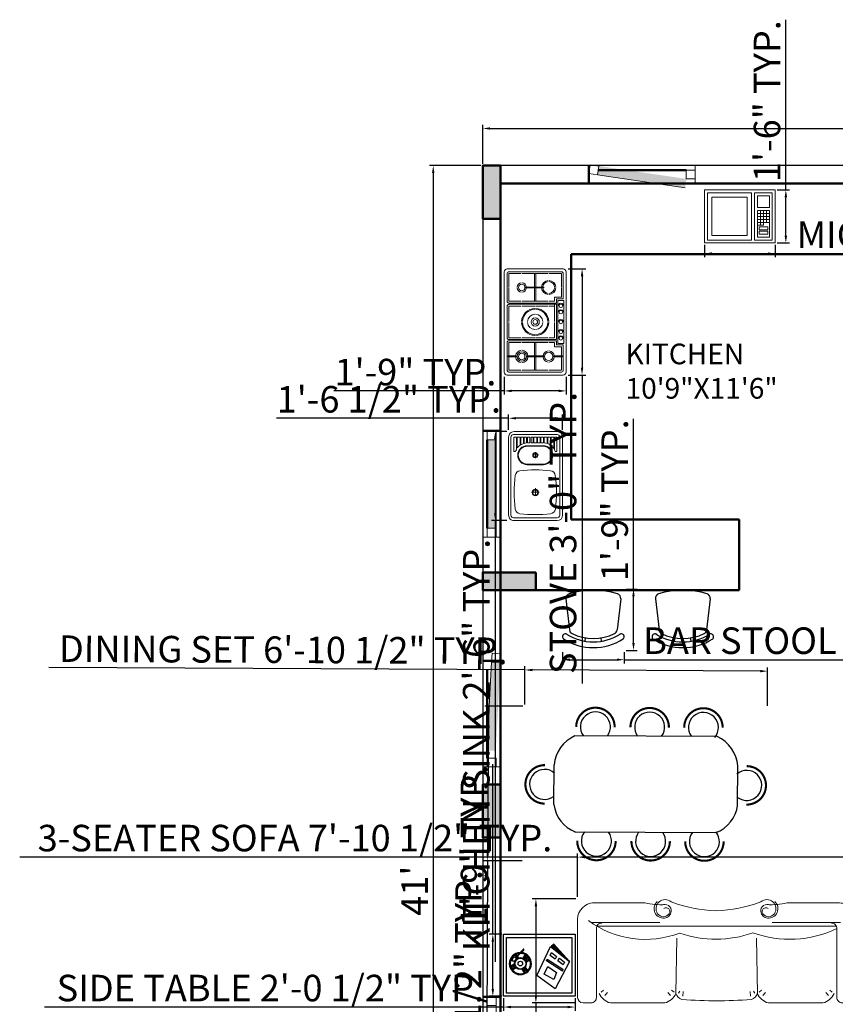
# Model space of a CAD drawing. Units: inches. Extents: x 3064 to 19385, y 846 to 15425.
# Tile 3 of 108: x 3064 to 3340, y 1112 to 1446. Entities that reach past the tile are written whole.
import ezdxf

# ---------------------------------------------------------------- set-up
doc = ezdxf.new("R2010")
doc.units = ezdxf.units.IN
for name, color, linetype, lineweight in [('A-ANNO-DIMS', 2, 'Continuous', 18), ('A-AREA-IDEN', 3, 'Continuous', 18), ('A-COLS', 1, 'Continuous', 35), ('A-EQPM', 8, 'Continuous', 18), ('A-FLOR-FIXT', 9, 'Continuous', 18), ('A-FURN', 8, 'Continuous', 18), ('A-GLAZ', 4, 'Continuous', 18), ('A-WALL', 7, 'Continuous', 50), ('C-PROP', 6, 'Continuous', 25)]:
    doc.layers.add(name, color=color, linetype=linetype, lineweight=lineweight)
for name, color, linetype in [('BLO', 135, 'Continuous'), ('FUR', 42, 'Continuous'), ('NOITHAT', 21, 'Continuous'), ('Win', 152, 'Continuous')]:
    doc.layers.add(name, color=color, linetype=linetype)
doc.styles.get("Standard").update_dxf_attribs({"font": 'arial.ttf'})
doc.dimstyles.new('ISO-25', dxfattribs={"dimtxt": 9, "dimasz": 2.5, "dimexe": 1.25, "dimexo": 0.625, "dimtad": 1, "dimdec": 1, "dimlunit": 3, "dimtxsty": 'Standard', "dimcen": 2.5, "dimadec": 0, "dimazin": 0, "dimtfac": 1, "dimtdec": 1, "dimtmove": 0, "dimatfit": 3, "dimfxl": 1, "dimarcsym": 0})

# ---------------------------------------------------------------- blocks, each defined once
blk = doc.blocks.new('din')
at = {"layer": 'FUR', "ltscale": 0.25}
for p, q in [((70.23, 15.24), (9.28, 15.24)), ((0, 3.44), (0, -13.56)), ((79.14, 3.44), (79.14, -13.56)), ((8.91, -26.16), (70.23, -26.16))]:
    blk.add_line(p, q, dxfattribs=at)
at = {"layer": 'FUR', "ltscale": 0.25, "const_width": 0.9}
for points in [[(22.5, 19.02, 1.012537), (5.94, 19.02, 1.012537)], [(45.67, 19.02, 1.012537), (29.11, 19.02, 1.012537)], [(69.02, 19.02, 1.012537), (52.46, 19.02, 1.012537)], [(-3.79, 3.1, 1.012537), (-3.79, -13.47, 1.012537)], [(83.08, 3.1, -1.012537), (83.08, -13.47, -1.012537)], [(23.18, -29.95, -1.012537), (6.61, -29.95, -1.012537)], [(46.34, -29.95, -1.012537), (29.78, -29.95, -1.012537)], [(69.7, -29.95, -1.012537), (53.14, -29.95, -1.012537)]]:
    blk.add_lwpolyline(points, format="xyb", dxfattribs=at)
at = {"layer": 'FUR', "ltscale": 0.25}
for centre, radius, start, end in [((14.22, 19.13), 6.48, 323.1301, 221.2163), ((37.39, 19.13), 6.48, 323.1301, 216.8699), ((60.74, 19.13), 6.48, 323.1301, 216.8699), ((14.55, 1.54), 14.67, 111.0491, 172.5731), ((64.59, 1.54), 14.67, 7.4269, 68.9509), ((-3.89, -5.18), 6.48, 53.1301, 311.2163), ((83.18, -5.18), 6.48, 228.7837, 126.8699), ((15.28, -12.21), 15.34, 185.0602, 245.4675), ((63.86, -12.21), 15.34, 294.5325, 354.9398), ((14.89, -30.05), 6.48, 138.7837, 36.8699), ((38.06, -30.05), 6.48, 143.1301, 36.8699), ((61.42, -30.05), 6.48, 143.1301, 36.8699)]:
    blk.add_arc(centre, radius, start, end, dxfattribs=at)
blk = doc.blocks.new('A$C558E769F')
at = {"layer": 'NOITHAT'}
for p, q in [((29.4, 426.4), (61.1, 154.1)), ((508.9, 426.4), (477.2, 154.1)), ((197.1, 55.9), (201.8, 84.2)), ((341.2, 55.9), (336.5, 84.2))]:
    blk.add_line(p, q, dxfattribs=at)
for centre, radius, start, end in [((69.1, 431), 40, 107.02981, 186.63805), ((269.2, -222), 723, 72.97019, 107.02981), ((469.2, 431), 40, 353.36195, 72.97019), ((25.3, 93.7), 25.7, 44.80366, 252.32262), ((269.2, 492.6), 442.6, 237.77056, 302.22944), ((100.8, 158.7), 40, 186.63805, 243.24485), ((269.2, 492.6), 413.9, 243.24485, 296.75515), ((437.5, 158.7), 40, 296.75515, 353.36195), ((513, 93.7), 25.7, 287.67738, 135.19634), ((269.2, 492.6), 492.6, 237.85101, 302.14899)]:
    blk.add_arc(centre, radius, start, end, dxfattribs=at)
blk = doc.blocks.new('sofa-32')
at = {"color": 0, "linetype": 'ByBlock'}
for p, q in [((-0.026, 0.9238), (-0.1, 0.9238)), ((0.657, 0.9252), (0.1531, 0.9252)), ((1.6158, 0.9252), (2.1197, 0.9252)), ((2.3728, 0.9238), (2.2988, 0.9238)), ((-0.15, 0.15), (-0.15, 0.8738)), ((0.024, 0.2361), (0.024, 0.8738)), ((0.05, 0.8375), (0.05, 0.8379)), ((0.0903, 0.8062), (0.0682, 0.8242)), ((0.1006, 0.8574), (0.1265, 0.8286)), ((0.7096, 0.8574), (0.6837, 0.8286)), ((0.7199, 0.8062), (0.742, 0.8242)), ((0.7682, 0.3257), (0.7597, 0.8384)), ((0.7601, 0.8375), (0.7601, 0.8379)), ((0.7823, 0.8346), (0.7966, 0.8162)), ((0.8227, 0.8633), (0.8259, 0.8195)), ((1.4501, 0.8633), (1.447, 0.8195)), ((1.4906, 0.8346), (1.4762, 0.8162)), ((1.5046, 0.3257), (1.5131, 0.8384)), ((1.5127, 0.8375), (1.5127, 0.8379)), ((1.5529, 0.8062), (1.5308, 0.8242)), ((1.5632, 0.8574), (1.5891, 0.8286)), ((2.1722, 0.8574), (2.1463, 0.8286)), ((2.1825, 0.8062), (2.2046, 0.8242)), ((2.2228, 0.8375), (2.2228, 0.8379)), ((2.2228, 0.8375), (2.2228, 0.8379)), ((2.2488, 0.2361), (2.2488, 0.8738)), ((2.4228, 0.15), (2.4228, 0.8738)), ((0.0289, 0.2145), (2.2439, 0.2145)), ((-0.01, 0.1801), (0.6238, 0.1801)), ((2.2948, 0.1801), (1.661, 0.1801)), ((0, 0), (0.4856, 0)), ((2.2848, 0), (1.7991, 0))]:
    blk.add_line(p, q, dxfattribs=at)
at = {"color": 0, "linetype": 'ByBlock', "extrusion": (0, 0, -1)}
for centre, major_axis, start_param, end_param in [((-0.1, 0.8738), (0.0354, 0.0354), 3.926992, 5.497787), ((-0.026, 0.8738), (-0.0354, 0.0354), 0.785398, 2.356196), ((0.1997, 0.7661), (0.1173, 0.1173), 4.372209, 5.213218), ((0.6105, 0.7661), (0.1173, 0.1173), -0.500829, 0.34018), ((1.6624, 0.7661), (0.1173, 0.1173), 4.372209, 5.213218), ((2.0731, 0.7661), (-0.1173, 0.1173), 1.069968, 1.910976), ((2.2988, 0.8738), (-0.0354, 0.0354), 5.497786, 7.068583), ((2.3728, 0.8738), (0.0354, 0.0354), -0.785398, 0.785398), ((0.8378, 0.8143), (-0.0573, 0.0573), 5.78837, 6.779907), ((1.1202, -2.7856), (2.6094, 2.6094), -0.86827, -0.778364), ((1.1526, -2.7856), (2.6094, 2.6094), -0.792432, -0.702526), ((1.435, 0.8143), (-0.0573, 0.0573), 1.074075, 2.065611), ((0.4599, -0.6685), (0.71, 0.71), 5.048761, 5.844539), ((1.7954, -0.5466), (-0.6249, 0.6249), 0.417642, 1.423136), ((1.1424, -0.6685), (-0.71, 0.71), 0.438646, 1.125824), ((0.074, 0.2361), (0.0354, 0.0354), 2.356194, 3.926992), ((2.1988, 0.2361), (0.0354, 0.0354), 0.785397, 2.356194), ((0, 0.15), (0.1061, 0.1061), 2.356194, 3.926992), ((0.6576, 0.0525), (-0.0624, 0.0624), 4.675944, 7.152385), ((0.6708, 0.0524), (-0.059, 0.059), 3.186406, 6.094039), ((0.6552, 0.0629), (0.0458, 0.0458), 4.523242, 6.472337), ((0.6801, 0.0798), (-0.0245, 0.0245), 1.759948, 4.523241), ((0.6592, 0.0712), (-0.0491, 0.0491), 0.8692, 2.230507), ((1.6256, 0.0712), (-0.0491, 0.0491), 5.623477, 6.984784), ((1.614, 0.0524), (0.059, 0.059), 0.189149, 3.096782), ((1.6047, 0.0798), (0.0245, 0.0245), 1.759947, 4.52324), ((1.6295, 0.0629), (0.0458, 0.0458), 4.52324, 6.472335), ((1.6271, 0.0525), (-0.0624, 0.0624), 0.701599, 3.17804), ((2.2728, 0.15), (0.1061, 0.1061), 0.785398, 2.356194), ((0.6324, -0.6613), (-0.479, 0.479), 0.566947, 0.842011), ((0.6701, 0.0726), (0.0414, 0.0414), 0.659711, 2.852687), ((1.2153, -1.3904), (1.0359, 1.0359), 5.158011, 5.447964), ((1.0694, -1.3904), (1.0359, 1.0359), 5.547613, 5.837566), ((1.6147, 0.0726), (-0.0414, 0.0414), 3.430501, 5.623477), ((1.6523, -0.6613), (0.479, 0.479), 5.441177, 5.716241)]:
    blk.add_ellipse(centre, major_axis=major_axis, ratio=1, start_param=start_param, end_param=end_param, dxfattribs=at)
blk = doc.blocks.new('sink 1')
for points in [[(5.86, 24.22), (-5.86, 24.22)], [(-7.34, 1.48), (-7.34, 22.73)], [(-6.56, 1.48), (-6.56, 22.73)], [(6.01, 23.43), (-5.86, 23.43)], [(6.72, 1.48), (6.72, 22.73)], [(7.34, 1.48), (7.34, 22.73)], [(1.09, 16.48), (-0.94, 16.48)], [(0, 15.39), (0, 17.42)], [(-2.09, 8.99), (2.28, 8.99)], [(-2.09, 8.84), (2.28, 8.84)], [(-5.78, 5.39), (-5.78, 5.39)], [(-5.31, 5.39), (-5.31, 5.39)], [(0.78, 6.33), (-0.78, 6.33)], [(0, 5.55), (0, 7.26)], [(5.94, 5.39), (5.94, 5.39)], [(-5.16, 4.92), (-5.16, 4.92)], [(-5, 1.48), (-5, 4.69)], [(-5, 1.48), (-4.22, 1.48), (-4.22, 3.83)], [(-4.84, 4.45), (-4.84, 4.45)], [(-4.22, 3.83), (-4.22, 3.83)], [(-4.06, 1.48), (-4.06, 3.69)], [(-4.06, 1.48), (-3.28, 1.48), (-3.28, 3.27)], [(-3.91, 3.52), (-3.91, 3.52)], [(-3.28, 3.2), (-3.28, 3.2)], [(-3.12, 3.2), (-3.12, 3.2)], [(-2.34, 3.05), (-2.34, 3.05)], [(-2.19, 3.05), (-2.19, 3.05)], [(-2.09, 3.99), (2.28, 3.99)], [(-2.09, 3.84), (2.28, 3.84)], [(-1.41, 3.05), (-1.41, 3.05)], [(-1.25, 3.05), (-1.25, 3.05)], [(-0.47, 1.48), (-1.25, 1.48), (-1.25, 3.05), (-0.47, 3.05)], [(-0.62, 3.05), (-0.62, 3.05)], [(-0.47, 1.48), (-0.47, 3.05)], [(-0.31, 3.05), (-0.31, 3.05)], [(0.47, 1.48), (-0.31, 1.48), (-0.31, 3.05), (0.47, 3.05)], [(0.31, 3.05), (0.31, 3.05)], [(0.47, 1.48), (0.47, 3.05)], [(0.62, 3.05), (0.62, 3.05)], [(1.25, 3.05), (1.25, 3.05)], [(1.56, 3.05), (1.56, 3.05)], [(2.19, 3.05), (2.19, 3.05)], [(2.5, 3.05), (2.5, 3.05)], [(3.12, 3.2), (3.12, 3.2)], [(3.28, 1.48), (4.06, 1.48), (4.06, 3.57)], [(3.28, 1.48), (3.28, 3.2)], [(3.44, 3.2), (3.44, 3.2)], [(4.06, 3.52), (4.06, 3.52)], [(4.22, 1.48), (4.22, 3.67)], [(4.37, 3.83), (4.37, 3.83)], [(5, 4.45), (5, 4.45)], [(5.16, 4.92), (5.16, 4.92)], [(6.01, 0.78), (-5.86, 0.78)], [(5.86, 0), (-5.86, 0)], [(-5.78, 1.48), (-5.78, 1.48)], [(-5.16, 1.48), (-5.16, 1.48)], [(-4.84, 1.48), (-4.84, 1.48)], [(-4.22, 1.48), (-4.22, 1.48)], [(-3.91, 1.48), (-3.91, 1.48)], [(-3.28, 1.48), (-3.28, 1.48)], [(-3.12, 1.48), (-3.12, 1.48)], [(-2.34, 1.48), (-2.34, 1.48)], [(-2.19, 1.48), (-2.19, 1.48)], [(-1.41, 1.48), (-1.41, 1.48)], [(-1.25, 1.48), (-1.25, 1.48)], [(-0.62, 1.48), (-0.62, 1.48)], [(-0.31, 1.48), (-0.31, 1.48)], [(0.31, 1.48), (0.31, 1.48)], [(0.62, 1.48), (0.62, 1.48)], [(1.25, 1.48), (1.25, 1.48)], [(1.56, 1.48), (1.56, 1.48)], [(2.19, 1.48), (2.19, 1.48)], [(2.5, 1.48), (2.5, 1.48)], [(3.12, 1.48), (3.12, 1.48)], [(3.44, 1.48), (3.44, 1.48)], [(4.06, 1.48), (4.06, 1.48)], [(4.37, 1.48), (4.37, 1.48)], [(5, 1.48), (5, 1.48)], [(5.16, 1.48), (5.16, 1.48)], [(5.94, 1.48), (5.94, 1.48)]]:
    blk.add_lwpolyline(points)
for points in [[(-5.16, 4.92), (-5.16, 1.48), (-5.78, 1.48), (-5.78, 5.39), (-5.31, 5.39, -0.068511), (-5.16, 4.92)], [(5.16, 4.92, 0.248301), (5.47, 5.39), (5.94, 5.39), (5.94, 1.48), (5.16, 1.48), (5.16, 4.92)], [(4.06, 3.57, -0.061679), (3.32, 3.22)], [(4.22, 1.48), (5, 1.48), (5, 4.45, -0.083542), (4.22, 3.67, -0.083542)]]:
    blk.add_lwpolyline(points, format="xyb")
for points in [[(-3.12, 3.22), (-3.12, 1.48), (-2.34, 1.48), (-2.34, 3.05, -0.06228)], [(2.5, 3.05), (2.5, 1.48), (3.12, 1.48), (3.12, 3.2, -0.050256)]]:
    blk.add_lwpolyline(points, format="xyb", close=True)
for points in [[(-2.19, 3.05), (-1.41, 3.05), (-1.41, 1.48), (-2.19, 1.48)], [(0.62, 3.05), (1.25, 3.05), (1.25, 1.48), (0.62, 1.48)], [(2.19, 1.48), (2.19, 3.05), (1.56, 3.05), (1.56, 1.48)]]:
    blk.add_lwpolyline(points, close=True)
for centre, radius in [((0.09, 16.57), 0.859), ((0.09, 16.57), 0.703), ((0.09, 6.41), 0.703), ((0.09, 6.41), 0.547)]:
    blk.add_circle(centre, radius)
for centre, radius, start, end in [((-5.86, 22.73), 1.48, 90, 180), ((5.86, 22.73), 1.48, 360, 90), ((-5.86, 22.73), 0.703, 90, 180), ((-3.87, 20.82), 1.53, 97.3256, 171.1849), ((0.09, -12.65), 35.23, 83.2159, 96.7841), ((4.06, 20.82), 1.53, 8.8151, 82.6744), ((6.01, 22.73), 0.703, 0, 90), ((30.19, 16.56), 35.85, 172.7947, 187.4213), ((-30, 16.56), 35.85, 352.5787, 7.2053), ((-3.89, 12.12), 1.48, 187.4212, 263.2159), ((4.08, 12.12), 1.48, 276.7841, 352.5788), ((-2.1, 6.41), 2.58, 90, 270), ((-2.1, 6.41), 2.42, 90, 270), ((0.09, 45.63), 35.23, 263.2159, 276.7841), ((2.28, 6.41), 2.58, 270, 90), ((2.28, 6.41), 2.42, 270, 90), ((-2.15, 6.48), 3.36, 212.1095, 232.0862), ((-2.1, 6.41), 3.36, 234.156, 249.3275), ((2.14, 6.36), 3.36, 289.8633, 290.5971), ((-5.86, 1.48), 1.48, 180, 270), ((-5.86, 1.48), 0.703, 180, 270), ((5.86, 1.48), 1.48, 270, 0), ((6.01, 1.48), 0.703, 270, 360)]:
    blk.add_arc(centre, radius, start, end)
blk = doc.blocks.new('STOVE')
for p, q in [((11.85, 19.7), (11.55, 19.7)), ((11.55, 16.92), (11.55, 19.7)), ((11.85, 16.92), (11.55, 16.92)), ((11.85, 16.92), (11.85, 19.7)), ((-11.85, 13.73), (-11.85, 7.62)), ((-11.85, 13.73), (-11.55, 13.73)), ((-11.55, 13.73), (-11.55, 7.62)), ((-11.85, 10.75), (-16.4, 10.75)), ((-11.85, 10.25), (-16.4, 10.25)), ((-7, 10.75), (-11.55, 10.75)), ((-7, 10.25), (-11.55, 10.25)), ((7, 10.75), (11.55, 10.75)), ((7, 10.25), (11.55, 10.25)), ((11.85, 13.23), (11.55, 13.23)), ((11.55, 13.23), (11.55, 7.57)), ((11.85, 13.23), (11.85, 7.57)), ((11.85, 10.75), (16.4, 10.75)), ((11.85, 10.25), (16.4, 10.25)), ((-11.85, 7.62), (-11.55, 7.62)), ((11.85, 7.57), (11.55, 7.57)), ((-7, 3.9), (-8.4, 3.9)), ((-5.4, 3.9), (-6, 3.9)), ((-5.4, 3.9), (-0.15, 3.9)), ((0.15, 3.9), (5.4, 3.9)), ((7, 3.9), (8.4, 3.9)), ((8.4, 3.9), (8.4, 1.6)), ((11.85, 4.28), (11.55, 4.28)), ((11.55, 4.28), (11.55, 1.3)), ((11.85, 4.28), (11.85, 1.3)), ((-7.8, 3.3), (-7.8, 1)), ((-6.4, 3.3), (-7.8, 3.3)), ((7.3, 2.8), (-7.3, 2.8)), ((-7.3, 2.8), (-7.3, 0.8)), ((7.3, 0.8), (-7.3, 0.8)), ((6.4, 3.3), (7.8, 3.3)), ((7.3, 2.8), (7.3, 0.8)), ((7.8, 3.3), (7.8, 1)), ((11.85, 1.3), (11.55, 1.3))]:
    blk.add_line(p, q)
for points in [[(-17, 21), (17, 21, -0.414214), (18, 20), (18, 1, -0.414214), (17, 0), (-17, 0, -0.414214), (-18, 1), (-18, 20, -0.414214)], [(6, 3.3), (-6, 3.3), (-6, 19.4, -0.414214), (-5.4, 20), (5.4, 20, -0.414214), (6, 19.4)]]:
    blk.add_lwpolyline(points, format="xyb", close=True)
for points in [[(-7.8, 1), (-16.4, 1, -0.414214), (-17, 1.6), (-17, 19.4, -0.414214), (-16.4, 20), (-7, 20, -0.414214), (-6.4, 19.4), (-6.4, 3.3)], [(6.4, 19.4, -0.414214), (7, 20), (16.4, 20, -0.414214), (17, 19.4), (17, 1.6, -0.414214), (16.4, 1), (7.8, 1)]]:
    blk.add_lwpolyline(points, format="xyb")
for points in [[(-16.4, 15.22), (-16.4, 19.4), (-11.85, 19.4)], [(-11.55, 19.4), (-7, 19.4), (-7, 15.22)], [(-5.4, 15.22), (-5.4, 19.4), (-0.15, 19.4)], [(0.15, 19.4), (5.4, 19.4), (5.4, 15.22)], [(6.4, 3.3), (6.4, 19.4)], [(7, 15.22), (7, 19.4), (11.55, 19.4)], [(11.85, 19.4), (16.4, 19.4), (16.4, 15.22)], [(-16.4, 6.08), (-16.4, 14.92)], [(-7, 14.92), (-7, 6.08)], [(-5.4, 10.65), (-5.4, 14.92)], [(5.4, 14.92), (5.4, 10.65)], [(7, 6.08), (7, 14.92)], [(16.4, 14.92), (16.4, 6.08)], [(-5.4, 6.08), (-5.4, 10.35)], [(5.4, 10.35), (5.4, 6.08)], [(-11.85, 1.6), (-16.4, 1.6), (-16.4, 5.77)], [(-8.4, 3.9), (-8.4, 1.6), (-11.55, 1.6)], [(-7, 5.77), (-7, 3.9)], [(-5.4, 3.9), (-5.4, 5.77)], [(5.4, 5.77), (5.4, 3.9)], [(7, 3.9), (7, 5.77)], [(16.4, 5.77), (16.4, 1.6), (11.85, 1.6)], [(11.55, 1.6), (8.4, 1.6)]]:
    blk.add_lwpolyline(points)
for centre, radius in [((-11.7, 15.07), 1.1), ((11.7, 15.07), 1.6), ((11.7, 15.07), 1.1), ((0, 10.5), 1.4), ((0, 10.5), 0.8), ((11.7, 5.93), 1.4), ((-5.49, 1.8), 0.6), ((-3.3, 1.8), 0.6), ((0, 1.8), 0.6), ((3.39, 1.8), 0.6), ((5.57, 1.8), 0.6)]:
    blk.add_circle(centre, radius)
for centre, radius, start, end in [((11.7, 15.07), 2.1, 94.096, 175.904), ((11.7, 15.07), 2.1, 4.096, 85.904), ((-11.7, 15.07), 1.6, 95.3794, 174.6206), ((-11.7, 15.07), 1.6, 185.3794, 264.6206), ((-11.7, 15.07), 1.6, 5.3794, 84.6206), ((-11.7, 15.07), 1.6, 275.3794, 354.6206), ((0, 10.5), 4.6, 91.8687, 178.1313), ((0, 10.5), 4.3, 91.9991, 178.0009), ((0, 10.5), 4.6, 1.8687, 88.1313), ((0, 10.5), 4.3, 1.9991, 88.0009), ((11.7, 15.07), 2.1, 184.096, 265.904), ((11.7, 15.07), 2.1, 274.096, 355.904), ((0, 10.5), 4.6, 181.8687, 268.1313), ((0, 10.5), 4.3, 181.9991, 268.0009), ((0, 10.5), 2.6, 93.3074, 176.6926), ((0, 10.5), 2.6, 183.3074, 266.6926), ((0, 10.5), 2.6, 3.3074, 86.6926), ((0, 10.5), 4.6, 271.8687, 358.1313), ((0, 10.5), 4.3, 271.9991, 358.0009), ((0, 10.5), 2.6, 273.3074, 356.6926), ((-11.7, 5.93), 2.4, 93.5833, 176.4167), ((-11.7, 5.93), 2, 94.3012, 175.6988), ((-11.7, 5.93), 2.4, 3.5833, 86.4167), ((-11.7, 5.93), 2, 4.3012, 85.6988), ((11.7, 5.93), 1.9, 94.5281, 175.4719), ((11.7, 5.93), 1.9, 4.5281, 85.4719), ((-11.7, 5.93), 2.4, 183.5833, 266.4167), ((-11.7, 5.93), 2, 184.3012, 265.6988), ((-11.7, 5.93), 2.4, 273.5833, 356.4167), ((-11.7, 5.93), 2, 274.3012, 355.6988), ((11.7, 5.93), 1.9, 184.5281, 265.4719), ((11.7, 5.93), 1.9, 274.5281, 355.4719), ((-5.49, 1.8), 0.846, 89.9979, 270), ((-3.3, 1.8), 0.846, 89.9979, 270), ((0, 1.8), 0.846, 89.9979, 270), ((3.39, 1.8), 0.846, 89.9979, 270), ((5.57, 1.8), 0.846, 89.9979, 270)]:
    blk.add_arc(centre, radius, start, end)
blk = doc.blocks.new('Microwave')
for p, q in [((19, 7), (19, 11)), ((20, 11), (20, 7)), ((21, 7), (21, 11)), ((18, 10), (22, 10)), ((22, 9), (18, 9)), ((18, 8), (22, 8)), ((22, 7), (18, 7)), ((19, 6), (19, 7)), ((20, 7), (20, 6)), ((20, 6), (18, 6))]:
    blk.add_line(p, q)
for points in [[(0, 0), (0, 18), (24, 18), (24, 0)], [(1, 1), (1, 17), (16, 17), (16, 1)], [(17, 1), (17, 17), (23, 17), (23, 1)], [(2.5, 2.5), (2.5, 15.5), (14.5, 15.5), (14.5, 2.5)], [(18, 12), (18, 16), (22, 16), (22, 12)], [(18, 2), (18, 11), (22, 11), (22, 2)], [(18.5, 4.5), (18.5, 5.5), (21.5, 5.5), (21.5, 4.5)], [(18.5, 3), (18.5, 4), (21.5, 4), (21.5, 3)]]:
    blk.add_lwpolyline(points, close=True)
blk = doc.blocks.new('*D38')
at = {"layer": 'A-ANNO-DIMS', "color": 0, "lineweight": -2, "transparency": 16777216}
for p, q in [((3220.85, 1396.96), (3220.85, 1410.2)), ((3562.85, 1396.96), (3562.85, 1410.2)), ((3223.35, 1408.95), (3560.35, 1408.95))]:
    blk.add_line(p, q, dxfattribs=at)
at = {"layer": 'A-ANNO-DIMS', "color": 0, "transparency": 16777216}
for points in [[(3223.35, 1409.36), (3223.35, 1408.53), (3220.85, 1408.95)], [(3560.35, 1409.36), (3560.35, 1408.53), (3562.85, 1408.95)]]:
    blk.add_solid(points, dxfattribs=at)
at = {"layer": 'Defpoints', "color": 0, "transparency": 16777216}
for p in [(3562.85, 1408.95), (3220.85, 1396.34), (3562.85, 1396.34)]:
    blk.add_point(p, dxfattribs=at)
at = {"layer": 'A-ANNO-DIMS', "color": 0, "transparency": 16777216, "insert": (3391.85, 1414.17), "char_height": 9, "attachment_point": 5}
blk.add_mtext('28\'-6"', dxfattribs=at)
blk = doc.blocks.new('*D39')
at = {"layer": 'A-ANNO-DIMS', "color": 0, "lineweight": -2, "transparency": 16777216}
for p, q in [((3220.22, 1396.34), (3202.78, 1396.34)), ((3204.03, 1393.84), (3204.03, 906.84)), ((3220.22, 904.34), (3202.78, 904.34))]:
    blk.add_line(p, q, dxfattribs=at)
at = {"layer": 'A-ANNO-DIMS', "color": 0, "transparency": 16777216}
for points in [[(3203.61, 1393.84), (3204.45, 1393.84), (3204.03, 1396.34)], [(3203.61, 906.84), (3204.45, 906.84), (3204.03, 904.34)]]:
    blk.add_solid(points, dxfattribs=at)
at = {"layer": 'Defpoints', "color": 0, "transparency": 16777216}
for p in [(3220.85, 1396.34), (3204.03, 904.34), (3220.85, 904.34)]:
    blk.add_point(p, dxfattribs=at)
at = {"layer": 'A-ANNO-DIMS', "color": 0, "transparency": 16777216, "insert": (3198.89, 1150.34), "char_height": 9, "attachment_point": 5, "rotation": 90}
blk.add_mtext("41'", dxfattribs=at)
blk = doc.blocks.new('ST1')
at = {"layer": 'BLO'}
for p, q in [((2.87, 1.65), (2.87, 24.72)), ((2.87, 24.72), (22.87, 24.72)), ((3.87, 2.65), (3.87, 23.72)), ((3.87, 23.72), (21.87, 23.72)), ((21.87, 23.72), (21.87, 2.65)), ((22.87, 24.72), (22.87, 1.65)), ((22.87, 1.65), (2.87, 1.65)), ((21.87, 2.65), (3.87, 2.65))]:
    blk.add_line(p, q, dxfattribs=at)
at = {"layer": 'Win'}
for p, q in [((12.55, 22.44), (12.13, 20.85)), ((12.55, 22.44), (13.25, 21.19)), ((12.69, 22.48), (13.4, 21.2)), ((11.4, 21.86), (12.09, 20.65)), ((11.51, 21.94), (12.19, 20.74)), ((11.57, 21.85), (13.19, 21.3)), ((14.51, 20.87), (14.54, 20.9)), ((14.64, 20.77), (14.67, 20.79)), ((15.43, 20.61), (15.22, 19.97)), ((15.22, 19.97), (15.71, 20.33)), ((15.27, 19.81), (15.82, 20.21)), ((15.37, 21.5), (15.64, 21.7)), ((15.41, 20.64), (17.8, 18.17)), ((15.46, 21.36), (15.76, 21.58)), ((15.54, 20.8), (16.34, 20.79)), ((15.54, 20.77), (18.02, 18.4)), ((15.76, 21.58), (15.55, 20.96)), ((17.88, 18.31), (15.58, 20.6)), ((15.87, 20.45), (16.34, 20.79)), ((15.99, 20.33), (16.41, 20.64)), ((10.46, 17.93), (11.6, 18.76)), ((10.53, 17.78), (11.65, 18.59)), ((10.53, 17.78), (12.23, 17.8)), ((11.59, 18.54), (11.11, 16.99)), ((11.11, 16.99), (12.23, 17.8)), ((11.23, 16.87), (12.37, 17.7)), ((13.9, 17.44), (14.58, 16.23)), ((14.03, 17.48), (14.71, 16.28)), ((14.09, 17.38), (15.67, 16.91)), ((15.04, 18.04), (14.71, 16.28)), ((14.97, 18.16), (15.67, 16.91)), ((15, 18.22), (15.87, 17.69)), ((15.13, 18.43), (16.01, 17.9)), ((15.14, 18.13), (15.77, 17.01)), ((5.28, 8.07), (9.58, 13.93)), ((9.58, 13.93), (18.91, 9.59)), ((8.3, 8.54), (10.02, 11.57)), ((10.02, 11.57), (12.5, 10.4)), ((12.5, 10.4), (10.58, 7.59)), ((10.98, 5.74), (14.34, 10.89)), ((14.87, 10.68), (11.67, 5.58)), ((18.91, 9.59), (14.09, 3.45)), ((14.34, 10.89), (14.87, 10.68)), ((14.86, 8.07), (16.06, 9.73)), ((16.06, 9.73), (17.01, 9.23)), ((14.09, 3.45), (5.28, 8.07)), ((10.58, 7.59), (8.3, 8.54)), ((13.06, 5.5), (14.27, 7.16)), ((15.21, 6.66), (13.91, 5.03)), ((14.09, 3.45), (19.17, 9.31)), ((14.09, 3.45), (19.44, 9.01)), ((14.09, 3.45), (19.64, 8.8)), ((14.09, 3.45), (19.77, 8.63)), ((14.27, 7.16), (15.21, 6.66)), ((15.7, 7.6), (14.86, 8.07)), ((17.01, 9.23), (15.7, 7.6)), ((11.67, 5.58), (10.98, 5.74)), ((13.91, 5.03), (13.06, 5.5))]:
    blk.add_line(p, q, dxfattribs=at)
for radius in [1.91, 1.75, 0.74]:
    blk.add_circle((13.43, 19.29), radius, dxfattribs=at)
for centre, radius, start, end in [((13.43, 19.29), 3.56, 1.5005, 355.5882), ((13.43, 19.29), 3.27, 6.8421, 0.252), ((15.21, 21.57), 0.956, 171.718, 281.8824), ((14.47, 21.69), 0.203, 96.3605, 174.3012), ((14.6, 20.95), 0.956, 349.0729, 98.9437), ((15.51, 20.66), 0.106, 78.1124, 194.2793), ((15.97, 17.77), 0.128, 220.7943, 60.0122), ((17.91, 18.29), 0.161, 227.8642, 43.7153)]:
    blk.add_arc(centre, radius, start, end, dxfattribs=at)
blk = doc.blocks.new('WIN-900-A')
h = blk.add_hatch(color=256)
h.dxf.hatch_style = 1
h.paths.add_polyline_path([(33, 0), (33, 3), (3, 3), (3, 0)])
blk.add_line((3, 0), (33, 0))
blk.add_lwpolyline([(3, 0), (0, 0), (0, 3), (3, 3)], close=True)
blk = doc.blocks.new('WIN-900')
blk.add_line((0, 0), (30, 0))
blk.add_lwpolyline([(30, 0), (30, 3), (33, 3), (33, 0)], close=True)
blk = doc.blocks.new('WIN-1900')
blk.add_line((3, 0), (3, 66))
blk.add_lwpolyline([(3, 66), (0, 66), (0, 69), (3, 69)], close=True)
blk = doc.blocks.new('*D409')
at = {"layer": 'A-ANNO-DIMS', "color": 0, "lineweight": -2, "transparency": 16777216}
for p, q in [((3247.88, 1231.24), (3247.88, 1227.47)), ((3268.83, 1231.24), (3268.83, 1227.47)), ((3250.38, 1228.72), (3266.33, 1228.72)), ((3268.83, 1228.72), (3402.5, 1228.72))]:
    blk.add_line(p, q, dxfattribs=at)
at = {"layer": 'A-ANNO-DIMS', "color": 0, "transparency": 16777216}
for points in [[(3250.38, 1229.14), (3250.38, 1228.3), (3247.88, 1228.72)], [(3266.33, 1229.14), (3266.33, 1228.3), (3268.83, 1228.72)]]:
    blk.add_solid(points, dxfattribs=at)
at = {"layer": 'Defpoints', "color": 0, "transparency": 16777216}
for p in [(3247.88, 1231.86), (3268.83, 1231.86), (3268.83, 1228.72)]:
    blk.add_point(p, dxfattribs=at)
at = {"layer": 'A-ANNO-DIMS', "color": 0, "transparency": 16777216, "insert": (3336.92, 1234), "char_height": 9, "attachment_point": 5}
blk.add_mtext('BAR STOOL 1\'-9" TYP.', dxfattribs=at)
blk = doc.blocks.new('*D410')
at = {"layer": 'A-ANNO-DIMS', "color": 0, "lineweight": -2, "transparency": 16777216}
for p, q in [((3271.98, 1252.68), (3271.98, 1310.44)), ((3269.46, 1252.68), (3273.23, 1252.68)), ((3271.98, 1234.36), (3271.98, 1250.18)), ((3269.46, 1231.86), (3273.23, 1231.86))]:
    blk.add_line(p, q, dxfattribs=at)
at = {"layer": 'A-ANNO-DIMS', "color": 0, "transparency": 16777216}
for points in [[(3271.56, 1250.18), (3272.39, 1250.18), (3271.98, 1252.68)], [(3271.56, 1234.36), (3272.39, 1234.36), (3271.98, 1231.86)]]:
    blk.add_solid(points, dxfattribs=at)
at = {"layer": 'Defpoints', "color": 0, "transparency": 16777216}
for p in [(3268.83, 1252.68), (3271.98, 1252.68), (3268.83, 1231.86)]:
    blk.add_point(p, dxfattribs=at)
at = {"layer": 'A-ANNO-DIMS', "color": 0, "transparency": 16777216, "insert": (3266.76, 1282.81), "char_height": 9, "attachment_point": 5, "rotation": 90}
blk.add_mtext('1\'-9" TYP.', dxfattribs=at)
blk = doc.blocks.new('*D413')
at = {"layer": 'A-ANNO-DIMS', "color": 0, "lineweight": -2, "transparency": 16777216}
for p, q in [((3235.16, 1225.24), (3073.59, 1226.05)), ((3235.1, 1213.52), (3235.16, 1226.49)), ((3317.39, 1213.11), (3317.46, 1226.08)), ((3314.95, 1224.84), (3237.66, 1225.23))]:
    blk.add_line(p, q, dxfattribs=at)
at = {"layer": 'A-ANNO-DIMS', "color": 0, "transparency": 16777216}
for points in [[(3237.66, 1225.64), (3237.66, 1224.81), (3235.16, 1225.24)], [(3314.95, 1225.26), (3314.95, 1224.42), (3317.45, 1224.83)]]:
    blk.add_solid(points, dxfattribs=at)
at = {"layer": 'Defpoints', "color": 0, "transparency": 16777216}
for p in [(3235.16, 1225.24), (3235.1, 1212.9), (3317.39, 1212.49)]:
    blk.add_point(p, dxfattribs=at)
at = {"layer": 'A-ANNO-DIMS', "color": 0, "transparency": 16777216, "insert": (3153.15, 1230.93), "char_height": 9, "attachment_point": 5, "rotation": 359.7135}
blk.add_mtext('DINING SET 6\'-10 1/2" TYP.', dxfattribs=at)
blk = doc.blocks.new('*D414')
at = {"layer": 'A-ANNO-DIMS', "color": 0, "lineweight": -2, "transparency": 16777216}
for p, q in [((3234.47, 1212.9), (3221.5, 1212.96)), ((3222.74, 1210.46), (3222.5, 1163)), ((3234.21, 1160.44), (3221.24, 1160.51)), ((3222.49, 1160.5), (3222.09, 1080.56))]:
    blk.add_line(p, q, dxfattribs=at)
at = {"layer": 'A-ANNO-DIMS', "color": 0, "transparency": 16777216}
for points in [[(3222.32, 1210.46), (3223.16, 1210.46), (3222.75, 1212.96)], [(3222.09, 1163), (3222.92, 1163), (3222.49, 1160.5)]]:
    blk.add_solid(points, dxfattribs=at)
at = {"layer": 'Defpoints', "color": 0, "transparency": 16777216}
for p in [(3235.1, 1212.9), (3222.49, 1160.5), (3234.83, 1160.44)]:
    blk.add_point(p, dxfattribs=at)
at = {"layer": 'A-ANNO-DIMS', "color": 0, "transparency": 16777216, "insert": (3217.01, 1119.31), "char_height": 9, "attachment_point": 5, "rotation": 89.7135}
blk.add_mtext('4\'-4 1/2" TYP.', dxfattribs=at)
blk = doc.blocks.new('*D417')
at = {"layer": 'A-ANNO-DIMS', "color": 0, "lineweight": -2, "transparency": 16777216}
for p, q in [((3253.02, 1148.22), (3253.02, 1162.99)), ((3347.35, 1148.22), (3347.35, 1162.99)), ((3253.02, 1161.74), (3063.75, 1161.74)), ((3344.85, 1161.74), (3255.52, 1161.74))]:
    blk.add_line(p, q, dxfattribs=at)
at = {"layer": 'A-ANNO-DIMS', "color": 0, "transparency": 16777216}
for points in [[(3255.52, 1162.16), (3255.52, 1161.32), (3253.02, 1161.74)], [(3344.85, 1162.16), (3344.85, 1161.32), (3347.35, 1161.74)]]:
    blk.add_solid(points, dxfattribs=at)
at = {"layer": 'Defpoints', "color": 0, "transparency": 16777216}
for p in [(3253.02, 1161.74), (3253.02, 1147.59), (3347.35, 1147.59)]:
    blk.add_point(p, dxfattribs=at)
at = {"layer": 'A-ANNO-DIMS', "color": 0, "transparency": 16777216, "insert": (3157.13, 1167.03), "char_height": 9, "attachment_point": 5}
blk.add_mtext('3-SEATER SOFA 7\'-10 1/2" TYP.', dxfattribs=at)
blk = doc.blocks.new('*D418')
at = {"layer": 'A-ANNO-DIMS', "color": 0, "lineweight": -2, "transparency": 16777216}
for p, q in [((3252.39, 1147.59), (3237.62, 1147.59)), ((3238.87, 1145.09), (3238.87, 1114.76)), ((3252.39, 1112.26), (3237.62, 1112.26)), ((3238.87, 1112.26), (3238.87, 1025.53))]:
    blk.add_line(p, q, dxfattribs=at)
at = {"layer": 'A-ANNO-DIMS', "color": 0, "transparency": 16777216}
for points in [[(3238.45, 1145.09), (3239.29, 1145.09), (3238.87, 1147.59)], [(3238.45, 1114.76), (3239.29, 1114.76), (3238.87, 1112.26)]]:
    blk.add_solid(points, dxfattribs=at)
at = {"layer": 'Defpoints', "color": 0, "transparency": 16777216}
for p in [(3253.02, 1147.59), (3238.87, 1112.26), (3253.02, 1112.26)]:
    blk.add_point(p, dxfattribs=at)
at = {"layer": 'A-ANNO-DIMS', "color": 0, "transparency": 16777216, "insert": (3233.59, 1067.64), "char_height": 9, "attachment_point": 5, "rotation": 90}
blk.add_mtext('2\'-11 1/2" TYP.', dxfattribs=at)
blk = doc.blocks.new('*D423')
at = {"layer": 'A-ANNO-DIMS', "color": 0, "lineweight": -2, "transparency": 16777216}
for p, q in [((3228.99, 1306.1), (3223.83, 1306.1)), ((3225.08, 1303.6), (3225.08, 1278.4)), ((3228.99, 1275.9), (3223.83, 1275.9)), ((3225.08, 1275.9), (3225.08, 1126.17))]:
    blk.add_line(p, q, dxfattribs=at)
at = {"layer": 'A-ANNO-DIMS', "color": 0, "transparency": 16777216}
for points in [[(3224.66, 1303.6), (3225.5, 1303.6), (3225.08, 1306.1)], [(3224.66, 1278.4), (3225.5, 1278.4), (3225.08, 1275.9)]]:
    blk.add_solid(points, dxfattribs=at)
at = {"layer": 'Defpoints', "color": 0, "transparency": 16777216}
for p in [(3229.61, 1306.1), (3225.08, 1275.9), (3229.61, 1275.9)]:
    blk.add_point(p, dxfattribs=at)
at = {"layer": 'A-ANNO-DIMS', "color": 0, "transparency": 16777216, "insert": (3219.8, 1199.79), "char_height": 9, "attachment_point": 5, "rotation": 90}
blk.add_mtext('KITCHEN SINK 2\'-6" TYP.', dxfattribs=at)
blk = doc.blocks.new('*D424')
at = {"layer": 'A-ANNO-DIMS', "color": 0, "lineweight": -2, "transparency": 16777216}
for p, q in [((3229.61, 1310.63), (3150.88, 1310.63)), ((3229.61, 1306.73), (3229.61, 1311.88)), ((3245.43, 1310.63), (3232.11, 1310.63)), ((3247.93, 1306.73), (3247.93, 1311.88))]:
    blk.add_line(p, q, dxfattribs=at)
at = {"layer": 'A-ANNO-DIMS', "color": 0, "transparency": 16777216}
for points in [[(3232.11, 1311.05), (3232.11, 1310.22), (3229.61, 1310.63)], [(3245.43, 1311.05), (3245.43, 1310.22), (3247.93, 1310.63)]]:
    blk.add_solid(points, dxfattribs=at)
at = {"layer": 'Defpoints', "color": 0, "transparency": 16777216}
for p in [(3229.61, 1310.63), (3229.61, 1306.1), (3247.93, 1306.1)]:
    blk.add_point(p, dxfattribs=at)
at = {"layer": 'A-ANNO-DIMS', "color": 0, "transparency": 16777216, "insert": (3188.99, 1315.91), "char_height": 9, "attachment_point": 5}
blk.add_mtext('1\'-6 1/2" TYP.', dxfattribs=at)
blk = doc.blocks.new('*D425')
at = {"layer": 'A-ANNO-DIMS', "color": 0, "lineweight": -2, "transparency": 16777216}
for p, q in [((3249.76, 1361.31), (3255.78, 1361.31)), ((3254.53, 1358.81), (3254.53, 1327.81)), ((3249.76, 1325.31), (3255.78, 1325.31)), ((3254.53, 1325.31), (3254.53, 1220.63))]:
    blk.add_line(p, q, dxfattribs=at)
at = {"layer": 'A-ANNO-DIMS', "color": 0, "transparency": 16777216}
for points in [[(3254.12, 1358.81), (3254.95, 1358.81), (3254.53, 1361.31)], [(3254.12, 1327.81), (3254.95, 1327.81), (3254.53, 1325.31)]]:
    blk.add_solid(points, dxfattribs=at)
at = {"layer": 'Defpoints', "color": 0, "transparency": 16777216}
for p in [(3249.13, 1361.31), (3249.13, 1325.31), (3254.53, 1325.31)]:
    blk.add_point(p, dxfattribs=at)
at = {"layer": 'A-ANNO-DIMS', "color": 0, "transparency": 16777216, "insert": (3249.25, 1271.72), "char_height": 9, "attachment_point": 5, "rotation": 90}
blk.add_mtext('STOVE 3\'-0" TYP.', dxfattribs=at)
blk = doc.blocks.new('*D426')
at = {"layer": 'A-ANNO-DIMS', "color": 0, "lineweight": -2, "transparency": 16777216}
for p, q in [((3228.13, 1324.69), (3228.13, 1318.66)), ((3249.13, 1324.69), (3249.13, 1318.66)), ((3228.13, 1319.91), (3170.37, 1319.91)), ((3246.63, 1319.91), (3230.63, 1319.91))]:
    blk.add_line(p, q, dxfattribs=at)
at = {"layer": 'A-ANNO-DIMS', "color": 0, "transparency": 16777216}
for points in [[(3230.63, 1320.33), (3230.63, 1319.5), (3228.13, 1319.91)], [(3246.63, 1320.33), (3246.63, 1319.5), (3249.13, 1319.91)]]:
    blk.add_solid(points, dxfattribs=at)
at = {"layer": 'Defpoints', "color": 0, "transparency": 16777216}
for p in [(3228.13, 1325.31), (3249.13, 1325.31), (3228.13, 1319.91)]:
    blk.add_point(p, dxfattribs=at)
at = {"layer": 'A-ANNO-DIMS', "color": 0, "transparency": 16777216, "insert": (3198, 1325.13), "char_height": 9, "attachment_point": 5}
blk.add_mtext('1\'-9" TYP.', dxfattribs=at)
blk = doc.blocks.new('*D427')
at = {"layer": 'A-ANNO-DIMS', "color": 0, "lineweight": -2, "transparency": 16777216}
for p, q in [((3296.06, 1369.47), (3296.06, 1365.25)), ((3298.56, 1366.5), (3317.56, 1366.5)), ((3320.06, 1369.47), (3320.06, 1365.25)), ((3320.06, 1366.5), (3460.68, 1366.5))]:
    blk.add_line(p, q, dxfattribs=at)
at = {"layer": 'A-ANNO-DIMS', "color": 0, "transparency": 16777216}
for points in [[(3298.56, 1366.92), (3298.56, 1366.08), (3296.06, 1366.5)], [(3317.56, 1366.92), (3317.56, 1366.08), (3320.06, 1366.5)]]:
    blk.add_solid(points, dxfattribs=at)
at = {"layer": 'Defpoints', "color": 0, "transparency": 16777216}
for p in [(3296.06, 1370.1), (3320.06, 1370.1), (3320.06, 1366.5)]:
    blk.add_point(p, dxfattribs=at)
at = {"layer": 'A-ANNO-DIMS', "color": 0, "transparency": 16777216, "insert": (3391.62, 1371.78), "char_height": 9, "attachment_point": 5}
blk.add_mtext('MICROWAVE 2\'-0" TYP.', dxfattribs=at)
blk = doc.blocks.new('*D428')
at = {"layer": 'A-ANNO-DIMS', "color": 0, "lineweight": -2, "transparency": 16777216}
for p, q in [((3323.66, 1388.1), (3323.66, 1445.86)), ((3320.68, 1388.1), (3324.91, 1388.1)), ((3323.66, 1372.6), (3323.66, 1385.6)), ((3320.68, 1370.1), (3324.91, 1370.1))]:
    blk.add_line(p, q, dxfattribs=at)
at = {"layer": 'A-ANNO-DIMS', "color": 0, "transparency": 16777216}
for points in [[(3323.24, 1385.6), (3324.08, 1385.6), (3323.66, 1388.1)], [(3323.24, 1372.6), (3324.08, 1372.6), (3323.66, 1370.1)]]:
    blk.add_solid(points, dxfattribs=at)
at = {"layer": 'Defpoints', "color": 0, "transparency": 16777216}
for p in [(3320.06, 1388.1), (3323.66, 1388.1), (3320.06, 1370.1)]:
    blk.add_point(p, dxfattribs=at)
at = {"layer": 'A-ANNO-DIMS', "color": 0, "transparency": 16777216, "insert": (3318.44, 1418.23), "char_height": 9, "attachment_point": 5, "rotation": 90}
blk.add_mtext('1\'-6" TYP.', dxfattribs=at)
blk = doc.blocks.new('*D429')
at = {"layer": 'A-ANNO-DIMS', "color": 0, "lineweight": -2, "transparency": 16777216}
for p, q in [((3227.89, 1113.89), (3227.89, 1109.62)), ((3252.16, 1113.89), (3252.16, 1109.62)), ((3227.89, 1110.87), (3072.19, 1110.87)), ((3249.66, 1110.87), (3230.39, 1110.87))]:
    blk.add_line(p, q, dxfattribs=at)
at = {"layer": 'A-ANNO-DIMS', "color": 0, "transparency": 16777216}
for points in [[(3230.39, 1111.29), (3230.39, 1110.46), (3227.89, 1110.87)], [(3249.66, 1111.29), (3249.66, 1110.46), (3252.16, 1110.87)]]:
    blk.add_solid(points, dxfattribs=at)
at = {"layer": 'Defpoints', "color": 0, "transparency": 16777216}
for p in [(3227.89, 1114.51), (3252.16, 1114.51), (3227.89, 1110.87)]:
    blk.add_point(p, dxfattribs=at)
at = {"layer": 'A-ANNO-DIMS', "color": 0, "transparency": 16777216, "insert": (3148.79, 1116.15), "char_height": 9, "attachment_point": 5}
blk.add_mtext('SIDE TABLE 2\'-0 1/2" TYP.', dxfattribs=at)
blk = doc.blocks.new('*D430')
at = {"layer": 'A-ANNO-DIMS', "color": 0, "lineweight": -2, "transparency": 16777216}
for p, q in [((3224.25, 1135.55), (3224.25, 1193.32)), ((3227.26, 1135.55), (3223, 1135.55)), ((3224.25, 1117.01), (3224.25, 1133.05)), ((3227.26, 1114.51), (3223, 1114.51))]:
    blk.add_line(p, q, dxfattribs=at)
at = {"layer": 'A-ANNO-DIMS', "color": 0, "transparency": 16777216}
for points in [[(3223.83, 1133.05), (3224.67, 1133.05), (3224.25, 1135.55)], [(3223.83, 1117.01), (3224.67, 1117.01), (3224.25, 1114.51)]]:
    blk.add_solid(points, dxfattribs=at)
at = {"layer": 'Defpoints', "color": 0, "transparency": 16777216}
for p in [(3224.25, 1135.55), (3227.89, 1135.55), (3227.89, 1114.51)]:
    blk.add_point(p, dxfattribs=at)
at = {"layer": 'A-ANNO-DIMS', "color": 0, "transparency": 16777216, "insert": (3219.03, 1165.68), "char_height": 9, "attachment_point": 5, "rotation": 90}
blk.add_mtext('1\'-9" TYP.', dxfattribs=at)

msp = doc.modelspace()

# ---------------------------------------------------------------- hatches: boundary and pattern name
at = {"layer": 'A-COLS'}
h = msp.add_hatch(color=256, dxfattribs=at)
h.dxf.hatch_style = 1
h.paths.add_polyline_path([(3220.85, 1378.34), (3226.85, 1378.34), (3226.85, 1396.34), (3220.85, 1396.34)])
h = msp.add_hatch(color=256, dxfattribs=at)
h.dxf.hatch_style = 1
h.paths.add_polyline_path([(3238.85, 1252.34), (3238.85, 1258.34), (3220.85, 1258.34), (3220.85, 1252.34)])
h = msp.add_hatch(color=256, dxfattribs=at)
h.dxf.hatch_style = 1
h.paths.add_polyline_path([(3220.85, 1168.34), (3226.85, 1168.34), (3226.85, 1186.34), (3220.85, 1186.34)])
at = {"layer": 'A-GLAZ'}
h = msp.add_hatch(color=256, dxfattribs=at)
h.dxf.hatch_style = 1
h.paths.add_polyline_path([(3222.35, 1273.34), (3225.35, 1273.34), (3225.35, 1303.34), (3222.35, 1303.34)])

# ---------------------------------------------------------------- linework, layer by layer
for p, q in [((3292.85, 1396.34), (3292.85, 1390.34)), ((3220.85, 1270.34), (3226.85, 1270.34)), ((3220.85, 1192.34), (3226.85, 1192.34))]:
    msp.add_line(p, q, dxfattribs=at)
for points in [[(3292.85, 1391.84), (3289.85, 1391.84), (3289.85, 1394.84), (3292.85, 1394.84)], [(3225.35, 1270.34), (3222.35, 1270.34), (3222.35, 1273.34), (3225.35, 1273.34)], [(3225.35, 1192.34), (3222.35, 1192.34), (3222.35, 1195.34), (3225.35, 1195.34)]]:
    msp.add_lwpolyline(points, close=True, dxfattribs=at)
at = {"layer": 'A-WALL'}
for p, q in [((3256.85, 1396.34), (3256.85, 1390.34)), ((3259.85, 1394.84), (3289.85, 1394.84)), ((3355.85, 1390.34), (3226.85, 1390.34)), ((3226.85, 1390.34), (3226.85, 982.34)), ((3355.85, 1366.34), (3250.85, 1366.34)), ((3250.85, 1366.34), (3250.85, 1276.34)), ((3220.85, 1306.34), (3226.85, 1306.34)), ((3222.35, 1303.34), (3222.35, 1273.34)), ((3250.85, 1276.34), (3307.85, 1276.34)), ((3307.85, 1276.34), (3307.85, 1252.34)), ((3226.85, 1252.34), (3307.85, 1252.34)), ((3220.85, 1228.34), (3226.85, 1228.34)), ((3222.35, 1225.34), (3222.35, 1195.34)), ((3226.85, 1114.34), (3220.85, 1114.34))]:
    msp.add_line(p, q, dxfattribs=at)
for points in [[(3226.85, 1378.34), (3226.85, 1396.34), (3220.85, 1396.34), (3220.85, 1378.34)], [(3238.85, 1258.34), (3220.85, 1258.34), (3220.85, 1252.34), (3238.85, 1252.34)], [(3226.85, 1168.34), (3226.85, 1186.34), (3220.85, 1186.34), (3220.85, 1168.34)]]:
    msp.add_lwpolyline(points, close=True, dxfattribs=at)
at = {"layer": 'C-PROP'}
for p, q in [((3562.85, 1396.34), (3220.85, 1396.34)), ((3220.85, 1396.34), (3220.85, 880.34))]:
    msp.add_line(p, q, dxfattribs=at)

# ---------------------------------------------------------------- block references
at = {"layer": 'A-EQPM'}
msp.add_blockref('Microwave', (3296.06, 1370.1), dxfattribs=at)
at = {"layer": 'A-EQPM', "xscale": -1, "rotation": 90}
msp.add_blockref('STOVE', (3249.13, 1343.31), dxfattribs=at)
at = {"layer": 'A-FLOR-FIXT', "xscale": 1.24732326381372, "yscale": 1.24732326381372, "zscale": 1.24732326381372, "rotation": 180}
msp.add_blockref('sink 1', (3238.77, 1306.1), dxfattribs=at)
at = {"layer": 'A-FURN', "xscale": 0.0387879515044038, "yscale": 0.0387879515044038, "zscale": 0.0387879515044038}
for p in [(3247.91, 1232.84), (3278.27, 1232.84)]:
    msp.add_blockref('A$C558E769F', p, dxfattribs=at)
at = {"layer": 'A-FURN'}
for name, p, xscale, yscale, zscale, rotation in [('din', (3307.31, 1182.01), 0.787402, 0.787402, 0.787402, 179.7134895170222), ('sofa-32', (3341.85, 1146.18), 36.66436083614781, 36.66436083614781, 36.66436083614781, 180), ('ST1', (3253.89, 1111.49), 1.051988476719542, 1.051988476719542, 1.051988476719542, 90)]:
    msp.add_blockref(name, p, dxfattribs=dict(at, xscale=xscale, yscale=yscale, zscale=zscale, rotation=rotation))
at = {"layer": 'A-GLAZ'}
for name, p, rotation in [('WIN-900-A', (3256.84, 1393.67), 351.6350998303229), ('WIN-900', (3225.35, 1273.34), 90.00000000000036), ('WIN-900-A', (3224.02, 1230.88), 266.9173551180347)]:
    msp.add_blockref(name, p, dxfattribs=dict(at, rotation=rotation))
msp.add_blockref('WIN-1900', (3222.35, 1045.34), dxfattribs=at)

# ---------------------------------------------------------------- texts
at = {"layer": 'A-AREA-IDEN', "insert": (3269.26, 1335.96), "char_height": 7, "attachment_point": 1}
msp.add_mtext_dynamic_manual_height_columns('KITCHEN\\P10\'9"X11\'6"', width=67.5924, gutter_width=12.5, heights=[0], dxfattribs=at)

# ---------------------------------------------------------------- dimensions: what is measured, and where the dimension line sits
at = {"layer": 'A-ANNO-DIMS'}
for base, p1, p2, angle, text, picture, middle in [((3323.66, 1388.1), (3320.06, 1370.1), (3320.06, 1388.1), 90, '<> TYP.', '*D428', (3318.44, 1418.23)), ((3254.53, 1325.31), (3249.13, 1361.31), (3249.13, 1325.31), 270, 'STOVE <> TYP.', '*D425', (3249.25, 1271.72)), ((3229.61, 1310.63), (3247.93, 1306.1), (3229.61, 1306.1), 180, '<> TYP.', '*D424', (3188.99, 1315.91)), ((3228.13, 1319.91), (3249.13, 1325.31), (3228.13, 1325.31), 180, '<> TYP.', '*D426', (3198, 1325.13)), ((3271.98, 1252.68), (3268.83, 1231.86), (3268.83, 1252.68), 90, '<> TYP.', '*D410', (3266.76, 1282.81)), ((3225.08, 1275.9), (3229.61, 1306.1), (3229.61, 1275.9), 270, 'KITCHEN SINK <> TYP.', '*D423', (3219.8, 1199.79)), ((3235.16, 1225.24), (3317.39, 1212.49), (3235.1, 1212.9), 179.7135, 'DINING SET <> TYP.', '*D413', (3153.15, 1230.93)), ((3222.49, 1160.5), (3235.1, 1212.9), (3234.83, 1160.44), 269.7135, '<> TYP.', '*D414', (3217.01, 1119.31)), ((3253.02, 1161.74), (3347.35, 1147.59), (3253.02, 1147.59), 180, '3-SEATER SOFA <> TYP.', '*D417', (3157.13, 1167.03)), ((3224.25, 1135.55), (3227.89, 1114.51), (3227.89, 1135.55), 90, '<> TYP.', '*D430', (3219.03, 1165.68)), ((3227.89, 1110.87), (3252.16, 1114.51), (3227.89, 1114.51), 180, 'SIDE TABLE <> TYP.', '*D429', (3148.79, 1116.15)), ((3238.87, 1112.26), (3253.02, 1147.59), (3253.02, 1112.26), 270, '<> TYP.', '*D418', (3233.59, 1067.64))]:
    dim = msp.add_linear_dim(base=base, p1=p1, p2=p2, angle=angle, text=text, dimstyle='ISO-25', override={"dimdec": 1, "dimrnd": 0, "dimzin": 1, "dimlunit": 4, "dimfrac": 2}, dxfattribs=at)
    dim.commit()
    dim.dimension.update_dxf_attribs({"geometry": picture, "text_midpoint": middle})
dim = msp.add_linear_dim(base=(3562.85, 1408.95), p1=(3220.85, 1396.34), p2=(3562.85, 1396.34), dimstyle='ISO-25', override={"dimclrd": 0, "dimclre": 0, "dimclrt": 0}, dxfattribs=at)
dim.commit()
dim.dimension.update_dxf_attribs({"geometry": '*D38', "text_midpoint": (3391.85, 1414.17)})
dim = msp.add_linear_dim(base=(3204.03, 904.34), p1=(3220.85, 1396.34), p2=(3220.85, 904.34), angle=90, dimstyle='ISO-25', override={"dimclrd": 0, "dimclre": 0, "dimclrt": 0}, dxfattribs=at)
dim.commit()
dim.dimension.update_dxf_attribs({"geometry": '*D39', "text_midpoint": (3198.89, 1150.34)})
for base, p1, p2, text, picture, middle in [((3320.06, 1366.5), (3296.06, 1370.1), (3320.06, 1370.1), 'MICROWAVE <> TYP.', '*D427', (3391.62, 1371.78)), ((3268.8322, 1228.7186), (3247.875, 1231.8622), (3268.8322, 1231.8622), 'BAR STOOL <> TYP.', '*D409', (3336.9156, 1234.0001))]:
    dim = msp.add_linear_dim(base=base, p1=p1, p2=p2, text=text, dimstyle='ISO-25', override={"dimdec": 1, "dimrnd": 0, "dimzin": 1, "dimlunit": 4, "dimfrac": 2}, dxfattribs=at)
    dim.commit()
    dim.dimension.update_dxf_attribs({"geometry": picture, "text_midpoint": middle})

doc.saveas('drawing.dxf')
